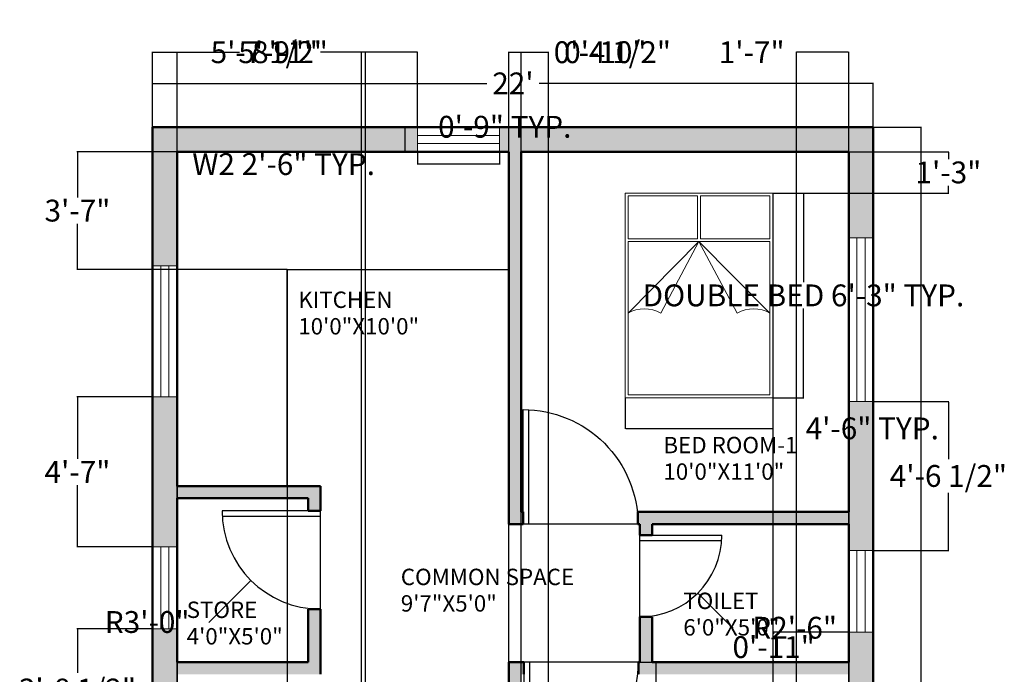
# Model space of a CAD drawing. Units: inches. Extents: x 23 to 387, y 67 to 650.
# Tile 3 of 3: x 23 to 384, y 410 to 650. Entities that reach past the tile are written whole.
import ezdxf

# ---------------------------------------------------------------- set-up
doc = ezdxf.new("R2010")
doc.units = ezdxf.units.IN
doc.header["$MEASUREMENT"] = 0
for name, color, linetype, lineweight in [('A-ANNO-DIMS', 4, 'Continuous', 18), ('A-AREA-IDEN', 4, 'Continuous', 25), ('A-DOOR', 41, 'Continuous', 25), ('A-FLOR-FIXT', 31, 'Continuous', 25), ('A-FURN', 31, 'Continuous', 18), ('A-GLAZ', 146, 'Continuous', 18), ('A-WALL', 240, 'Continuous', 50), ('A-WALL-PATT', 31, 'Continuous', 13)]:
    doc.layers.add(name, color=color, linetype=linetype, lineweight=lineweight)
doc.styles.get("Standard").update_dxf_attribs({"font": 'italic8.shx'})
doc.dimstyles.get("Standard").update_dxf_attribs({"dimtxt": 8, "dimasz": 0.18, "dimexe": 0.18, "dimexo": 0.0625, "dimgap": 0.09, "dimtad": 0, "dimtih": 1, "dimtoh": 1, "dimdec": 1, "dimzin": 0, "dimdsep": 46, "dimlunit": 3, "dimtxsty": 'Standard', "dimcen": 0.09, "dimadec": 0, "dimazin": 0, "dimtfac": 1, "dimtdec": 1, "dimtofl": 0, "dimtmove": 0, "dimatfit": 3, "dimfxl": 1, "dimtolj": 1, "dimtzin": 0, "dimarcsym": 0})

# ---------------------------------------------------------------- blocks, each defined once
blk = doc.blocks.new('*D4')
at = {"layer": 'A-ANNO-DIMS', "color": 0, "lineweight": -2, "transparency": 16777216}
for p, q in [((71.8, 610.61), (71.8, 626.8)), ((71.98, 626.62), (194.19, 626.62)), ((335.62, 626.62), (213.41, 626.62)), ((335.8, 610.61), (335.8, 626.8))]:
    blk.add_line(p, q, dxfattribs=at)
at = {"layer": 'A-ANNO-DIMS', "color": 0, "transparency": 16777216}
for points in [[(71.98, 626.65), (71.98, 626.59), (71.8, 626.62)], [(335.62, 626.65), (335.62, 626.59), (335.8, 626.62)]]:
    blk.add_solid(points, dxfattribs=at)
at = {"layer": 'Defpoints', "color": 0, "transparency": 16777216}
for p in [(335.8, 626.62), (71.8, 610.55), (335.8, 610.55)]:
    blk.add_point(p, dxfattribs=at)
at = {"layer": 'A-ANNO-DIMS', "color": 0, "transparency": 16777216, "insert": (203.8, 626.62), "char_height": 8, "attachment_point": 5}
blk.add_mtext("\\A1;22'", dxfattribs=at)
blk = doc.blocks.new('*D5')
at = {"layer": 'A-ANNO-DIMS', "color": 0, "lineweight": -2, "transparency": 16777216}
for p, q in [((335.86, 610.55), (353.42, 610.55)), ((353.24, 610.37), (353.24, 375.4)), ((353.24, 130.73), (353.24, 365.7)), ((335.86, 130.55), (353.42, 130.55))]:
    blk.add_line(p, q, dxfattribs=at)
at = {"layer": 'A-ANNO-DIMS', "color": 0, "transparency": 16777216}
for points in [[(353.21, 610.37), (353.27, 610.37), (353.24, 610.55)], [(353.21, 130.73), (353.27, 130.73), (353.24, 130.55)]]:
    blk.add_solid(points, dxfattribs=at)
at = {"layer": 'Defpoints', "color": 0, "transparency": 16777216}
for p in [(335.8, 610.55), (335.8, 130.55), (353.24, 130.55)]:
    blk.add_point(p, dxfattribs=at)
at = {"layer": 'A-ANNO-DIMS', "color": 0, "transparency": 16777216, "insert": (353.24, 370.55), "char_height": 8, "attachment_point": 5}
blk.add_mtext("\\A1;40'", dxfattribs=at)
blk = doc.blocks.new('BED-DOUBLE')
for p, q in [((26.5, 58.27), (26.5, 74)), ((27.5, 58.27), (27.5, 74)), ((1, 58.27), (26.5, 58.27)), ((27.5, 58.27), (53, 58.27)), ((1, 57.27), (53, 57.27)), ((27, 57.27), (1, 30.99)), ((13, 30.99), (27, 57.27)), ((27, 57.27), (53, 30.99)), ((41, 30.99), (27, 57.27))]:
    blk.add_line(p, q)
blk.add_lwpolyline([(54, 75), (0, 75), (0, 0), (54, 0)], close=True)
for points in [[(26.5, 74), (1, 74), (1, 58.27)], [(53, 58.27), (53, 74), (27.5, 74)], [(1, 57.27), (1, 1), (53, 1), (53, 57.27)]]:
    blk.add_lwpolyline(points)
for centre in [(7, 20.75), (47, 20.75)]:
    blk.add_arc(centre, 11.86, 59.6151, 120.3849)
blk = doc.blocks.new('DOOR-SWING-42IN')
for p, q in [((42, 42), (0, 42)), ((0, 42), (0, 0)), ((2, 42), (2, 0.05))]:
    blk.add_line(p, q)
blk.add_arc((0, 42), 42, 270, 0)
blk = doc.blocks.new('WIN-60IN')
for p, q in [((0, 0), (0, 60)), ((0, 60), (9, 60)), ((3, 0), (3, 60)), ((6, 0), (6, 60)), ((9, 60), (9, 0)), ((9, 0), (0, 0)), ((0, 0), (4.5, 0))]:
    blk.add_line(p, q)
blk = doc.blocks.new('WIN-30IN')
for p, q in [((0, 0), (0, 30)), ((0, 30), (9, 30)), ((3, 0), (3, 30)), ((6, 0), (6, 30)), ((9, 30), (9, 0)), ((9, 0), (0, 0)), ((0, 0), (4.5, 0))]:
    blk.add_line(p, q)
blk = doc.blocks.new('WIN-48IN')
for p, q in [((0, 0), (0, 48)), ((0, 48), (9, 48)), ((3, 0), (3, 48)), ((6, 0), (6, 48)), ((9, 48), (9, 0)), ((9, 0), (0, 0)), ((0, 0), (4.5, 0))]:
    blk.add_line(p, q)
blk = doc.blocks.new('*D14')
at = {"layer": 'A-ANNO-DIMS', "color": 0, "lineweight": -2, "transparency": 16777216}
for p, q in [((168.85, 601.49), (168.85, 596.87)), ((198.85, 601.49), (198.85, 596.87)), ((168.85, 597.05), (168.67, 597.05)), ((198.67, 597.05), (169.03, 597.05))]:
    blk.add_line(p, q, dxfattribs=at)
at = {"layer": 'A-ANNO-DIMS', "color": 0, "transparency": 16777216}
for points in [[(169.03, 597.08), (169.03, 597.02), (168.85, 597.05)], [(198.67, 597.08), (198.67, 597.02), (198.85, 597.05)]]:
    blk.add_solid(points, dxfattribs=at)
at = {"layer": 'Defpoints', "color": 0, "transparency": 16777216}
for p in [(168.85, 601.55), (198.85, 601.55), (168.85, 597.05)]:
    blk.add_point(p, dxfattribs=at)
at = {"layer": 'A-ANNO-DIMS', "color": 0, "transparency": 16777216, "insert": (119.81, 597.05), "char_height": 8, "attachment_point": 5}
blk.add_mtext('\\A1;W2 2\'-6" TYP.', dxfattribs=at)
blk = doc.blocks.new('*D15')
at = {"layer": 'A-ANNO-DIMS', "color": 0, "lineweight": -2, "transparency": 16777216}
for p, q in [((168.78, 610.55), (164.17, 610.55)), ((164.35, 610.55), (164.35, 610.73)), ((164.35, 610.73), (164.53, 610.73)), ((164.35, 601.73), (164.35, 610.37)), ((168.78, 601.55), (164.17, 601.55))]:
    blk.add_line(p, q, dxfattribs=at)
at = {"layer": 'A-ANNO-DIMS', "color": 0, "transparency": 16777216}
for points in [[(164.32, 610.37), (164.38, 610.37), (164.35, 610.55)], [(164.32, 601.73), (164.38, 601.73), (164.35, 601.55)]]:
    blk.add_solid(points, dxfattribs=at)
at = {"layer": 'Defpoints', "color": 0, "transparency": 16777216}
for p in [(164.35, 610.55), (168.85, 610.55), (168.85, 601.55)]:
    blk.add_point(p, dxfattribs=at)
at = {"layer": 'A-ANNO-DIMS', "color": 0, "transparency": 16777216, "insert": (200.81, 610.73), "char_height": 8, "attachment_point": 5}
blk.add_mtext('\\A1;0\'-9" TYP.', dxfattribs=at)
blk = doc.blocks.new('*D18')
at = {"layer": 'A-ANNO-DIMS', "color": 0, "lineweight": -2, "transparency": 16777216}
for p, q in [((299.01, 586.43), (310.38, 586.43)), ((310.2, 586.25), (310.2, 553.78)), ((310.2, 511.61), (310.2, 544.07)), ((299.01, 511.43), (310.38, 511.43))]:
    blk.add_line(p, q, dxfattribs=at)
at = {"layer": 'A-ANNO-DIMS', "color": 0, "transparency": 16777216}
for points in [[(310.17, 586.25), (310.23, 586.25), (310.2, 586.43)], [(310.17, 511.61), (310.23, 511.61), (310.2, 511.43)]]:
    blk.add_solid(points, dxfattribs=at)
at = {"layer": 'Defpoints', "color": 0, "transparency": 16777216}
for p in [(298.95, 586.43), (310.2, 586.43), (298.95, 511.43)]:
    blk.add_point(p, dxfattribs=at)
at = {"layer": 'A-ANNO-DIMS', "color": 0, "transparency": 16777216, "insert": (310.2, 548.93), "char_height": 8, "attachment_point": 5}
blk.add_mtext('\\A1;DOUBLE BED 6\'-3" TYP.', dxfattribs=at)
blk = doc.blocks.new('*D19')
at = {"layer": 'A-ANNO-DIMS', "color": 0, "lineweight": -2, "transparency": 16777216}
for p, q in [((244.95, 511.36), (244.95, 500)), ((298.95, 511.36), (298.95, 500)), ((245.13, 500.18), (298.77, 500.18)), ((298.95, 500.18), (299.13, 500.18))]:
    blk.add_line(p, q, dxfattribs=at)
at = {"layer": 'A-ANNO-DIMS', "color": 0, "transparency": 16777216}
for points in [[(245.13, 500.21), (245.13, 500.15), (244.95, 500.18)], [(298.77, 500.21), (298.77, 500.15), (298.95, 500.18)]]:
    blk.add_solid(points, dxfattribs=at)
at = {"layer": 'Defpoints', "color": 0, "transparency": 16777216}
for p in [(244.95, 511.43), (298.95, 511.43), (298.95, 500.18)]:
    blk.add_point(p, dxfattribs=at)
at = {"layer": 'A-ANNO-DIMS', "color": 0, "transparency": 16777216, "insert": (335.41, 500.18), "char_height": 8, "attachment_point": 5}
blk.add_mtext('\\A1;4\'-6" TYP.', dxfattribs=at)
blk = doc.blocks.new('*D21')
at = {"layer": 'A-ANNO-DIMS', "color": 0, "lineweight": -2, "transparency": 16777216}
for p, q in [((249.89, 414.55), (256.3, 414.55)), ((256.12, 414.37), (256.12, 398.4)), ((256.12, 372.73), (256.12, 388.7)), ((249.89, 372.55), (256.3, 372.55))]:
    blk.add_line(p, q, dxfattribs=at)
at = {"layer": 'A-ANNO-DIMS', "color": 0, "transparency": 16777216}
for points in [[(256.09, 414.37), (256.15, 414.37), (256.12, 414.55)], [(256.09, 372.73), (256.15, 372.73), (256.12, 372.55)]]:
    blk.add_solid(points, dxfattribs=at)
at = {"layer": 'Defpoints', "color": 0, "transparency": 16777216}
for p in [(249.82, 414.55), (256.12, 414.55), (249.82, 372.55)]:
    blk.add_point(p, dxfattribs=at)
at = {"layer": 'A-ANNO-DIMS', "color": 0, "transparency": 16777216, "insert": (256.12, 393.55), "char_height": 8, "attachment_point": 5}
blk.add_mtext('\\A1;3\'-6" TYP.', dxfattribs=at)
blk = doc.blocks.new('*D27')
at = {"layer": 'A-ANNO-DIMS', "color": 0, "lineweight": -2, "transparency": 16777216}
for p, q in [((71.8, 610.61), (71.8, 638.23)), ((71.98, 638.05), (103.66, 638.05)), ((168.67, 638.05), (136.98, 638.05)), ((168.85, 610.61), (168.85, 638.23))]:
    blk.add_line(p, q, dxfattribs=at)
at = {"layer": 'A-ANNO-DIMS', "color": 0, "transparency": 16777216}
for points in [[(71.98, 638.08), (71.98, 638.02), (71.8, 638.05)], [(168.67, 638.08), (168.67, 638.02), (168.85, 638.05)]]:
    blk.add_solid(points, dxfattribs=at)
at = {"layer": 'Defpoints', "color": 0, "transparency": 16777216}
for p in [(168.85, 638.05), (71.8, 610.55), (168.85, 610.55)]:
    blk.add_point(p, dxfattribs=at)
at = {"layer": 'A-ANNO-DIMS', "color": 0, "transparency": 16777216, "insert": (120.32, 638.05), "char_height": 8, "attachment_point": 5}
blk.add_mtext('\\A1;8\'-1"', dxfattribs=at)
blk = doc.blocks.new('*D29')
at = {"layer": 'A-ANNO-DIMS', "color": 0, "lineweight": -2, "transparency": 16777216}
for p, q in [((71.74, 511.71), (44.12, 511.71)), ((44.3, 511.53), (44.3, 489.07)), ((44.3, 456.92), (44.3, 479.37)), ((71.74, 456.74), (44.12, 456.74))]:
    blk.add_line(p, q, dxfattribs=at)
at = {"layer": 'A-ANNO-DIMS', "color": 0, "transparency": 16777216}
for points in [[(44.27, 511.53), (44.33, 511.53), (44.3, 511.71)], [(44.27, 456.92), (44.33, 456.92), (44.3, 456.74)]]:
    blk.add_solid(points, dxfattribs=at)
at = {"layer": 'Defpoints', "color": 0, "transparency": 16777216}
for p in [(71.8, 511.71), (44.3, 456.74), (71.8, 456.74)]:
    blk.add_point(p, dxfattribs=at)
at = {"layer": 'A-ANNO-DIMS', "color": 0, "transparency": 16777216, "insert": (44.3, 484.22), "char_height": 8, "attachment_point": 5}
blk.add_mtext('\\A1;4\'-7"', dxfattribs=at)
blk = doc.blocks.new('*D30')
at = {"layer": 'A-ANNO-DIMS', "color": 0, "lineweight": -2, "transparency": 16777216}
for p, q in [((71.74, 426.74), (44.12, 426.74)), ((44.3, 426.56), (44.3, 410.65)), ((44.3, 382.38), (44.3, 398.28)), ((71.74, 382.2), (44.12, 382.2))]:
    blk.add_line(p, q, dxfattribs=at)
at = {"layer": 'A-ANNO-DIMS', "color": 0, "transparency": 16777216}
for points in [[(44.27, 426.56), (44.33, 426.56), (44.3, 426.74)], [(44.27, 382.38), (44.33, 382.38), (44.3, 382.2)]]:
    blk.add_solid(points, dxfattribs=at)
at = {"layer": 'Defpoints', "color": 0, "transparency": 16777216}
for p in [(71.8, 426.74), (44.3, 382.2), (71.8, 382.2)]:
    blk.add_point(p, dxfattribs=at)
at = {"layer": 'A-ANNO-DIMS', "color": 0, "transparency": 16777216, "insert": (44.3, 404.47), "char_height": 8, "attachment_point": 5}
blk.add_mtext('\\A1;3\'-8 1/2"', dxfattribs=at)
blk = doc.blocks.new('*D33')
at = {"layer": 'A-ANNO-DIMS', "color": 0, "lineweight": -2, "transparency": 16777216}
for p, q in [((335.86, 510), (363.48, 510)), ((363.3, 509.82), (363.3, 488.93)), ((363.3, 455.67), (363.3, 476.56)), ((335.86, 455.49), (363.48, 455.49))]:
    blk.add_line(p, q, dxfattribs=at)
at = {"layer": 'A-ANNO-DIMS', "color": 0, "transparency": 16777216}
for points in [[(363.27, 509.82), (363.33, 509.82), (363.3, 510)], [(363.27, 455.67), (363.33, 455.67), (363.3, 455.49)]]:
    blk.add_solid(points, dxfattribs=at)
at = {"layer": 'Defpoints', "color": 0, "transparency": 16777216}
for p in [(335.8, 510), (335.8, 455.49), (363.3, 455.49)]:
    blk.add_point(p, dxfattribs=at)
at = {"layer": 'A-ANNO-DIMS', "color": 0, "transparency": 16777216, "insert": (363.3, 482.75), "char_height": 8, "attachment_point": 5}
blk.add_mtext('\\A1;4\'-6 1/2"', dxfattribs=at)
blk = doc.blocks.new('*D34')
at = {"layer": 'A-ANNO-DIMS', "color": 0, "lineweight": -2, "transparency": 16777216}
for p, q in [((326.74, 425.49), (299.12, 425.49)), ((299.3, 425.31), (299.3, 424.87)), ((299.3, 414.73), (299.3, 415.17)), ((326.74, 414.55), (299.12, 414.55))]:
    blk.add_line(p, q, dxfattribs=at)
at = {"layer": 'A-ANNO-DIMS', "color": 0, "transparency": 16777216}
for points in [[(299.27, 425.31), (299.33, 425.31), (299.3, 425.49)], [(299.27, 414.73), (299.33, 414.73), (299.3, 414.55)]]:
    blk.add_solid(points, dxfattribs=at)
at = {"layer": 'Defpoints', "color": 0, "transparency": 16777216}
for p in [(299.3, 425.49), (326.8, 425.49), (326.8, 414.55)]:
    blk.add_point(p, dxfattribs=at)
at = {"layer": 'A-ANNO-DIMS', "color": 0, "transparency": 16777216, "insert": (299.3, 420.02), "char_height": 8, "attachment_point": 5}
blk.add_mtext('\\A1;0\'-11"', dxfattribs=at)
blk = doc.blocks.new('*D37')
at = {"layer": 'A-ANNO-DIMS', "color": 0, "lineweight": -2, "transparency": 16777216}
for p, q in [((80.8, 139.61), (80.8, 638.23)), ((80.98, 638.05), (81.51, 638.05)), ((148.12, 638.05), (147.59, 638.05)), ((148.3, 139.61), (148.3, 638.23))]:
    blk.add_line(p, q, dxfattribs=at)
at = {"layer": 'A-ANNO-DIMS', "color": 0, "transparency": 16777216}
for points in [[(80.98, 638.08), (80.98, 638.02), (80.8, 638.05)], [(148.12, 638.08), (148.12, 638.02), (148.3, 638.05)]]:
    blk.add_solid(points, dxfattribs=at)
at = {"layer": 'Defpoints', "color": 0, "transparency": 16777216}
for p in [(148.3, 638.05), (80.8, 139.55), (148.3, 139.55)]:
    blk.add_point(p, dxfattribs=at)
at = {"layer": 'A-ANNO-DIMS', "color": 0, "transparency": 16777216, "insert": (114.55, 638.05), "char_height": 8, "attachment_point": 5}
blk.add_mtext('\\A1;5\'-7 1/2"', dxfattribs=at)
blk = doc.blocks.new('*D38')
at = {"layer": 'A-ANNO-DIMS', "color": 0, "lineweight": -2, "transparency": 16777216}
for p, q in [((80.8, 274.61), (80.8, 638.23)), ((80.98, 638.05), (97.28, 638.05)), ((149.58, 638.05), (133.27, 638.05)), ((149.76, 274.61), (149.76, 638.23))]:
    blk.add_line(p, q, dxfattribs=at)
at = {"layer": 'A-ANNO-DIMS', "color": 0, "transparency": 16777216}
for points in [[(80.98, 638.08), (80.98, 638.02), (80.8, 638.05)], [(149.58, 638.08), (149.58, 638.02), (149.76, 638.05)]]:
    blk.add_solid(points, dxfattribs=at)
at = {"layer": 'Defpoints', "color": 0, "transparency": 16777216}
for p in [(149.76, 638.05), (80.8, 274.55), (149.76, 274.55)]:
    blk.add_point(p, dxfattribs=at)
at = {"layer": 'A-ANNO-DIMS', "color": 0, "transparency": 16777216, "insert": (115.28, 638.05), "char_height": 8, "attachment_point": 5}
blk.add_mtext('\\A1;5\'-9"', dxfattribs=at)
blk = doc.blocks.new('*D39')
at = {"layer": 'A-ANNO-DIMS', "color": 0, "lineweight": -2, "transparency": 16777216}
for p, q in [((206.8, 192.11), (206.8, 638.23)), ((206.98, 638.05), (216.62, 638.05)), ((216.8, 192.11), (216.8, 638.23)), ((216.8, 638.05), (216.98, 638.05))]:
    blk.add_line(p, q, dxfattribs=at)
at = {"layer": 'A-ANNO-DIMS', "color": 0, "transparency": 16777216}
for points in [[(206.98, 638.08), (206.98, 638.02), (206.8, 638.05)], [(216.62, 638.08), (216.62, 638.02), (216.8, 638.05)]]:
    blk.add_solid(points, dxfattribs=at)
at = {"layer": 'Defpoints', "color": 0, "transparency": 16777216}
for p in [(216.8, 638.05), (206.8, 192.05), (216.8, 192.05)]:
    blk.add_point(p, dxfattribs=at)
at = {"layer": 'A-ANNO-DIMS', "color": 0, "transparency": 16777216, "insert": (237.64, 638.05), "char_height": 8, "attachment_point": 5}
blk.add_mtext('\\A1;0\'-10"', dxfattribs=at)
blk = doc.blocks.new('*D40')
at = {"layer": 'A-ANNO-DIMS', "color": 0, "lineweight": -2, "transparency": 16777216}
for p, q in [((80.8, 601.49), (80.8, 78.87)), ((121.14, 558.4), (121.14, 78.87)), ((80.8, 79.05), (80.62, 79.05)), ((120.96, 79.05), (80.98, 79.05))]:
    blk.add_line(p, q, dxfattribs=at)
at = {"layer": 'A-ANNO-DIMS', "color": 0, "transparency": 16777216}
for points in [[(80.98, 79.08), (80.98, 79.02), (80.8, 79.05)], [(120.96, 79.08), (120.96, 79.02), (121.14, 79.05)]]:
    blk.add_solid(points, dxfattribs=at)
at = {"layer": 'Defpoints', "color": 0, "transparency": 16777216}
for p in [(80.8, 601.55), (121.14, 558.46), (80.8, 79.05)]:
    blk.add_point(p, dxfattribs=at)
at = {"layer": 'A-ANNO-DIMS', "color": 0, "transparency": 16777216, "insert": (47.39, 79.05), "char_height": 8, "attachment_point": 5}
blk.add_mtext('\\A1;3\'-4 1/2"', dxfattribs=at)
blk = doc.blocks.new('*D41')
at = {"layer": 'A-ANNO-DIMS', "color": 0, "lineweight": -2, "transparency": 16777216}
for p, q in [((80.74, 601.55), (44.12, 601.55)), ((44.3, 601.37), (44.3, 584.86)), ((44.3, 558.64), (44.3, 575.15)), ((121.07, 558.46), (44.12, 558.46))]:
    blk.add_line(p, q, dxfattribs=at)
at = {"layer": 'A-ANNO-DIMS', "color": 0, "transparency": 16777216}
for points in [[(44.27, 601.37), (44.33, 601.37), (44.3, 601.55)], [(44.27, 558.64), (44.33, 558.64), (44.3, 558.46)]]:
    blk.add_solid(points, dxfattribs=at)
at = {"layer": 'Defpoints', "color": 0, "transparency": 16777216}
for p in [(80.8, 601.55), (44.3, 558.46), (121.14, 558.46)]:
    blk.add_point(p, dxfattribs=at)
at = {"layer": 'A-ANNO-DIMS', "color": 0, "transparency": 16777216, "insert": (44.3, 580), "char_height": 8, "attachment_point": 5}
blk.add_mtext('\\A1;3\'-7"', dxfattribs=at)
blk = doc.blocks.new('*D42')
at = {"layer": 'A-ANNO-DIMS', "color": 0, "lineweight": -2, "transparency": 16777216}
for p, q in [((202.3, 274.61), (202.3, 638.23)), ((202.48, 638.05), (206.62, 638.05)), ((206.8, 274.61), (206.8, 638.23)), ((206.8, 638.05), (206.98, 638.05))]:
    blk.add_line(p, q, dxfattribs=at)
at = {"layer": 'A-ANNO-DIMS', "color": 0, "transparency": 16777216}
for points in [[(202.48, 638.08), (202.48, 638.02), (202.3, 638.05)], [(206.62, 638.08), (206.62, 638.02), (206.8, 638.05)]]:
    blk.add_solid(points, dxfattribs=at)
at = {"layer": 'Defpoints', "color": 0, "transparency": 16777216}
for p in [(206.8, 638.05), (202.3, 274.55), (206.8, 274.55)]:
    blk.add_point(p, dxfattribs=at)
at = {"layer": 'A-ANNO-DIMS', "color": 0, "transparency": 16777216, "insert": (240.21, 638.05), "char_height": 8, "attachment_point": 5}
blk.add_mtext('\\A1;0\'-4 1/2"', dxfattribs=at)
blk = doc.blocks.new('*D43')
at = {"layer": 'A-ANNO-DIMS', "color": 0, "lineweight": -2, "transparency": 16777216}
for p, q in [((326.8, 601.49), (326.8, 78.87)), ((298.95, 586.36), (298.95, 78.87)), ((298.95, 79.05), (298.77, 79.05)), ((326.62, 79.05), (299.13, 79.05))]:
    blk.add_line(p, q, dxfattribs=at)
at = {"layer": 'A-ANNO-DIMS', "color": 0, "transparency": 16777216}
for points in [[(299.13, 79.08), (299.13, 79.02), (298.95, 79.05)], [(326.62, 79.08), (326.62, 79.02), (326.8, 79.05)]]:
    blk.add_solid(points, dxfattribs=at)
at = {"layer": 'Defpoints', "color": 0, "transparency": 16777216}
for p in [(326.8, 601.55), (298.95, 586.43), (298.95, 79.05)]:
    blk.add_point(p, dxfattribs=at)
at = {"layer": 'A-ANNO-DIMS', "color": 0, "transparency": 16777216, "insert": (280.78, 79.05), "char_height": 8, "attachment_point": 5}
blk.add_mtext('\\A1;2\'-4"', dxfattribs=at)
blk = doc.blocks.new('*D44')
at = {"layer": 'A-ANNO-DIMS', "color": 0, "lineweight": -2, "transparency": 16777216}
for p, q in [((326.86, 601.55), (363.48, 601.55)), ((363.3, 601.37), (363.3, 598.84)), ((363.3, 586.61), (363.3, 589.14)), ((299.01, 586.43), (363.48, 586.43))]:
    blk.add_line(p, q, dxfattribs=at)
at = {"layer": 'A-ANNO-DIMS', "color": 0, "transparency": 16777216}
for points in [[(363.27, 601.37), (363.33, 601.37), (363.3, 601.55)], [(363.27, 586.61), (363.33, 586.61), (363.3, 586.43)]]:
    blk.add_solid(points, dxfattribs=at)
at = {"layer": 'Defpoints', "color": 0, "transparency": 16777216}
for p in [(326.8, 601.55), (298.95, 586.43), (363.3, 586.43)]:
    blk.add_point(p, dxfattribs=at)
at = {"layer": 'A-ANNO-DIMS', "color": 0, "transparency": 16777216, "insert": (363.3, 593.99), "char_height": 8, "attachment_point": 5}
blk.add_mtext('\\A1;1\'-3"', dxfattribs=at)
blk = doc.blocks.new('*D45')
at = {"layer": 'A-ANNO-DIMS', "color": 0, "lineweight": -2, "transparency": 16777216}
for p, q in [((307.71, 638.05), (307.53, 638.05)), ((307.71, 290.5), (307.71, 638.23)), ((326.62, 638.05), (307.89, 638.05)), ((326.8, 274.61), (326.8, 638.23))]:
    blk.add_line(p, q, dxfattribs=at)
at = {"layer": 'A-ANNO-DIMS', "color": 0, "transparency": 16777216}
for points in [[(307.89, 638.08), (307.89, 638.02), (307.71, 638.05)], [(326.62, 638.08), (326.62, 638.02), (326.8, 638.05)]]:
    blk.add_solid(points, dxfattribs=at)
at = {"layer": 'Defpoints', "color": 0, "transparency": 16777216}
for p in [(307.71, 638.05), (307.71, 290.44), (326.8, 274.55)]:
    blk.add_point(p, dxfattribs=at)
at = {"layer": 'A-ANNO-DIMS', "color": 0, "transparency": 16777216, "insert": (291.25, 638.05), "char_height": 8, "attachment_point": 5}
blk.add_mtext('\\A1;1\'-7"', dxfattribs=at)
blk = doc.blocks.new('*D48')
at = {"layer": 'A-ANNO-DIMS', "color": 0, "lineweight": -2, "transparency": 16777216}
for p, q in [((133.21, 469.95), (133.39, 469.95)), ((133.3, 469.86), (133.3, 470.04)), ((92.57, 429.22), (107.72, 444.36)), ((92.39, 429.22), (92.57, 429.22))]:
    blk.add_line(p, q, dxfattribs=at)
at = {"layer": 'A-ANNO-DIMS', "color": 0, "transparency": 16777216}
blk.add_solid([(107.69, 444.39), (107.74, 444.34), (107.84, 444.49)], dxfattribs=at)
at = {"layer": 'Defpoints', "color": 0, "transparency": 16777216}
for p in [(133.3, 469.95), (107.84, 444.49)]:
    blk.add_point(p, dxfattribs=at)
at = {"layer": 'A-ANNO-DIMS', "color": 0, "transparency": 16777216, "insert": (69.82, 429.22), "char_height": 8, "attachment_point": 5}
blk.add_mtext('\\A1;R3\'-0"', dxfattribs=at)
blk = doc.blocks.new('*D49')
at = {"layer": 'A-ANNO-DIMS', "color": 0, "lineweight": -2, "transparency": 16777216}
for p, q in [((250.21, 461.06), (250.39, 461.06)), ((250.3, 460.97), (250.3, 461.15)), ((284.24, 427.12), (271.64, 439.72)), ((284.42, 427.12), (284.24, 427.12))]:
    blk.add_line(p, q, dxfattribs=at)
at = {"layer": 'A-ANNO-DIMS', "color": 0, "transparency": 16777216}
blk.add_solid([(271.66, 439.74), (271.62, 439.7), (271.51, 439.85)], dxfattribs=at)
at = {"layer": 'Defpoints', "color": 0, "transparency": 16777216}
for p in [(250.3, 461.06), (271.51, 439.85)]:
    blk.add_point(p, dxfattribs=at)
at = {"layer": 'A-ANNO-DIMS', "color": 0, "transparency": 16777216, "insert": (306.99, 427.12), "char_height": 8, "attachment_point": 5}
blk.add_mtext('\\A1;R2\'-6"', dxfattribs=at)

msp = doc.modelspace()

# ---------------------------------------------------------------- hatches: boundary and pattern name
at = {"layer": 'A-WALL-PATT'}
h = msp.add_hatch(color=256, dxfattribs=at)
h.dxf.hatch_style = 1
h.paths.add_polyline_path([(80.8, 601.55), (168.85, 601.55), (168.85, 610.55), (71.8, 610.55), (71.8, 559.71), (80.8, 559.71)])
h.paths.add_polyline_path([(335.8, 610.55), (198.85, 610.55), (198.85, 601.55), (202.3, 601.55), (202.3, 481.55), (202.3, 465.05), (207.59, 465.05), (207.59, 469.55), (206.8, 469.55), (206.8, 601.55), (326.8, 601.55), (326.8, 570), (331.3, 570), (335.8, 570)])
h.paths.add_polyline_path([(335.8, 510), (326.8, 510), (326.8, 469.55), (249.59, 469.55), (249.59, 465.05), (250.3, 465.05), (250.3, 461.06), (254.8, 461.06), (254.8, 465.05), (326.8, 465.05), (326.8, 455.49), (335.8, 455.49)])
h.paths.add_polyline_path([(335.8, 425.49), (326.8, 425.49), (326.8, 414.55), (254.8, 414.55), (254.8, 431.06), (250.3, 431.06), (250.3, 414.55), (249.82, 414.55), (249.82, 410.05), (326.8, 410.05), (326.8, 362.57), (335.8, 362.57)])
h.paths.add_polyline_path([(335.8, 302.57), (326.8, 302.57), (326.8, 274.55), (206.8, 274.55), (206.8, 410.05), (207.82, 410.05), (207.82, 414.55), (202.3, 414.55), (202.3, 274.55), (197.76, 274.55), (197.76, 270.05), (326.8, 270.05), (326.8, 253.25), (335.8, 253.25)])
h.paths.add_polyline_path([(335.8, 217.25), (326.8, 217.25), (326.8, 192.05), (202.3, 192.05), (202.3, 139.55), (196.3, 139.55), (196.3, 130.55), (206.8, 130.55), (206.8, 187.55), (335.8, 187.55)])
h.paths.add_polyline_path([(80.8, 203.04), (71.8, 203.04), (71.8, 130.55), (148.3, 130.55), (148.3, 139.55), (80.8, 139.55)])
h.paths.add_polyline_path([(80.8, 322.2), (71.8, 322.2), (71.8, 251.04), (80.8, 251.04), (80.8, 270.05), (149.76, 270.05), (149.76, 274.55), (80.8, 274.55)])
h.paths.add_polyline_path([(80.8, 410.05), (133.3, 410.05), (133.3, 433.95), (128.8, 433.95), (128.8, 414.55), (80.8, 414.55), (80.8, 426.74), (71.8, 426.74), (71.8, 382.2), (80.8, 382.2)])
h.paths.add_polyline_path([(133.3, 479.05), (80.8, 479.05), (80.8, 511.71), (71.8, 511.71), (71.8, 456.74), (80.8, 456.74), (80.8, 474.55), (128.8, 474.55), (128.8, 469.95), (133.3, 469.95)])
h.paths.add_polyline_path([(82.53, 419.2), (134.1, 419.2), (134.1, 429.92), (82.53, 429.92)], flags=9)

# ---------------------------------------------------------------- linework, layer by layer
at = {"layer": 'A-DOOR'}
for p, q in [((133.3, 469.95), (97.3, 469.95)), ((133.3, 433.95), (133.3, 469.95)), ((133.3, 467.95), (97.35, 467.95)), ((250.3, 431.06), (250.3, 461.06)), ((250.3, 461.06), (280.3, 461.06)), ((250.3, 459.06), (280.23, 459.06))]:
    msp.add_line(p, q, dxfattribs=at)
for centre, radius, start, end in [((133.3, 469.95), 36, 180, 270), ((250.3, 461.06), 30, 270, 0)]:
    msp.add_arc(centre, radius, start, end, dxfattribs=at)
at = {"layer": 'A-FLOR-FIXT'}
for p, q in [((121.14, 479.05), (121.14, 558.46)), ((121.14, 558.46), (202.3, 558.46))]:
    msp.add_line(p, q, dxfattribs=at)
at = {"layer": 'A-WALL'}
for p, q in [((335.8, 610.55), (71.8, 610.55)), ((71.8, 610.55), (71.8, 130.55)), ((335.8, 130.55), (335.8, 610.55)), ((80.8, 601.55), (80.8, 479.05)), ((202.3, 601.55), (80.8, 601.55)), ((202.3, 481.55), (202.3, 601.55)), ((326.8, 601.55), (206.8, 601.55)), ((206.8, 469.55), (206.8, 601.55)), ((326.8, 469.55), (326.8, 601.55)), ((202.3, 465.05), (202.3, 481.55)), ((80.8, 479.05), (133.3, 479.05)), ((133.3, 479.05), (133.3, 469.95)), ((80.8, 474.55), (80.8, 414.55)), ((80.8, 474.55), (128.8, 474.55)), ((128.8, 474.55), (128.8, 469.95)), ((128.8, 469.95), (133.3, 469.95)), ((207.59, 469.55), (206.8, 469.55)), ((207.59, 465.05), (207.59, 469.55)), ((326.8, 469.55), (249.59, 469.55)), ((249.59, 465.05), (249.59, 469.55)), ((207.59, 465.05), (202.3, 465.05)), ((250.3, 465.05), (249.59, 465.05)), ((250.3, 461.06), (250.3, 465.05)), ((326.8, 465.05), (254.8, 465.05)), ((254.8, 461.06), (254.8, 465.05)), ((326.8, 414.55), (326.8, 465.05)), ((250.3, 461.06), (254.8, 461.06)), ((128.8, 433.95), (133.3, 433.95)), ((128.8, 433.95), (128.8, 414.55)), ((133.3, 433.95), (133.3, 410.05)), ((250.3, 414.55), (250.3, 431.06)), ((250.3, 431.06), (254.8, 431.06)), ((254.8, 414.55), (254.8, 431.06)), ((80.8, 414.55), (128.8, 414.55)), ((202.3, 414.55), (207.82, 414.55)), ((202.3, 274.55), (202.3, 414.55)), ((207.82, 414.55), (207.82, 410.05)), ((249.82, 414.55), (249.82, 410.05)), ((249.82, 414.55), (250.3, 414.55)), ((254.8, 414.55), (326.8, 414.55))]:
    msp.add_line(p, q, dxfattribs=at)

# ---------------------------------------------------------------- block references
at = {"layer": 'A-DOOR', "extrusion": (0, 0, -1), "zscale": -1, "rotation": 180}
msp.add_blockref('DOOR-SWING-42IN', (-207.59, 507.05), dxfattribs=at)
at = {"layer": 'A-DOOR'}
msp.add_blockref('DOOR-SWING-42IN', (207.82, 372.55), dxfattribs=at)
at = {"layer": 'A-FURN'}
msp.add_blockref('BED-DOUBLE', (244.95, 511.43), dxfattribs=at)
at = {"layer": 'A-GLAZ', "rotation": 90.00000000000028}
msp.add_blockref('WIN-30IN', (198.85, 601.55), dxfattribs=at)
at = {"layer": 'A-GLAZ', "extrusion": (0, 0, -1), "zscale": -1, "rotation": 180}
msp.add_blockref('WIN-60IN', (-326.8, 570), dxfattribs=at)
at = {"layer": 'A-GLAZ'}
for name, p in [('WIN-48IN', (71.8, 511.71)), ('WIN-30IN', (71.8, 426.73)), ('WIN-30IN', (326.8, 425.49))]:
    msp.add_blockref(name, p, dxfattribs=at)

# ---------------------------------------------------------------- texts
at = {"layer": 'A-AREA-IDEN'}
for s, p in [('KITCHEN', (125.18, 544.33)), ('10\'0"X10\'0"', (125.18, 534.61)), ('BED ROOM-1', (258.92, 491.07)), ('10\'0"X11\'0"', (258.92, 481.35)), ('COMMON SPACE', (162.73, 442.75)), ('TOILET', (266.2, 433.98)), ('STORE', (84.31, 430.7)), ('9\'7"X5\'0"', (162.73, 433.04)), ('6\'0"X5\'0"', (266.2, 424.26)), ('4\'0"X5\'0"', (84.31, 420.99))]:
    msp.add_text(s, height=6, dxfattribs=at).set_placement(p)

# ---------------------------------------------------------------- dimensions: what is measured, and where the dimension line sits
at = {"layer": 'A-ANNO-DIMS'}
for base, p1, p2, override, picture, middle in [((148.3, 638.05), (80.8, 139.55), (148.3, 139.55), {"dimdec": 1, "dimlfac": 1, "dimrnd": 0, "dimzin": 1, "dimdsep": 46, "dimlunit": 4, "dimfrac": 2}, '*D37', (114.55, 638.05)), ((206.8, 638.05), (202.3, 274.55), (206.8, 274.55), {"dimdec": 1, "dimlfac": 1, "dimrnd": 0, "dimzin": 1, "dimdsep": 46, "dimlunit": 4, "dimfrac": 2}, '*D42', (240.21, 638.05)), ((168.8451, 638.049), (71.7992, 610.549), (168.8451, 610.549), {"dimdec": 1, "dimlfac": 1, "dimrnd": 0, "dimzin": 1, "dimdsep": 46, "dimlunit": 4, "dimfrac": 2}, '*D27', (120.3222, 638.049)), ((149.76, 638.05), (80.8, 274.55), (149.76, 274.55), {"dimdec": 1, "dimlfac": 1, "dimrnd": 0, "dimzin": 1, "dimdsep": 46, "dimlunit": 4, "dimfrac": 2}, '*D38', (115.28, 638.05)), ((216.8, 638.05), (206.8, 192.05), (216.8, 192.05), {"dimdec": 1, "dimlfac": 1, "dimrnd": 0, "dimzin": 1, "dimdsep": 46, "dimlunit": 4, "dimfrac": 2}, '*D39', (237.64, 638.05)), ((307.71, 638.05), (326.8, 274.55), (307.71, 290.44), {"dimdec": 1, "dimlfac": 1, "dimrnd": 0, "dimzin": 1, "dimdsep": 46, "dimlunit": 4, "dimfrac": 2}, '*D45', (291.25, 638.05)), ((335.8, 626.62), (71.8, 610.55), (335.8, 610.55), {"dimclrd": 0, "dimclre": 0, "dimclrt": 0}, '*D4', (203.8, 626.62)), ((80.8, 79.05), (121.14, 558.46), (80.8, 601.55), {"dimdec": 1, "dimlfac": 1, "dimrnd": 0, "dimzin": 1, "dimdsep": 46, "dimlunit": 4, "dimfrac": 2}, '*D40', (47.39, 79.05)), ((298.9524, 79.049), (326.7992, 601.549), (298.9524, 586.4268), {"dimdec": 1, "dimlfac": 1, "dimrnd": 0, "dimzin": 1, "dimdsep": 46, "dimlunit": 4, "dimfrac": 2}, '*D43', (280.7776, 79.049))]:
    dim = msp.add_linear_dim(base=base, p1=p1, p2=p2, dimstyle='Standard', override=override, dxfattribs=at)
    dim.commit()
    dim.dimension.update_dxf_attribs({"geometry": picture, "text_midpoint": middle})
for base, p1, p2, angle, text, picture, middle in [((164.35, 610.55), (168.85, 601.55), (168.85, 610.55), 90, '<> TYP.', '*D15', (200.81, 610.73)), ((168.85, 597.05), (198.85, 601.55), (168.85, 601.55), 180, 'W2 <> TYP.', '*D14', (119.81, 597.05)), ((310.2, 586.43), (298.95, 511.43), (298.95, 586.43), 90, 'DOUBLE BED <> TYP.', '*D18', (310.2, 548.93)), ((256.12, 414.55), (249.82, 372.55), (249.82, 414.55), 90, '<> TYP.', '*D21', (256.12, 393.55))]:
    dim = msp.add_linear_dim(base=base, p1=p1, p2=p2, angle=angle, text=text, dimstyle='Standard', override={"dimdec": 1, "dimlfac": 1, "dimrnd": 0, "dimzin": 1, "dimdsep": 46, "dimlunit": 4, "dimfrac": 2}, dxfattribs=at)
    dim.commit()
    dim.dimension.update_dxf_attribs({"geometry": picture, "text_midpoint": middle})
for base, p1, p2, override, picture, middle in [((353.24, 130.55), (335.8, 610.55), (335.8, 130.55), {"dimclrd": 0, "dimclre": 0, "dimclrt": 0}, '*D5', (353.24, 370.55)), ((44.3, 558.46), (80.8, 601.55), (121.14, 558.46), {"dimdec": 1, "dimlfac": 1, "dimrnd": 0, "dimzin": 1, "dimdsep": 46, "dimlunit": 4, "dimfrac": 2}, '*D41', (44.3, 580)), ((363.3, 586.43), (326.8, 601.55), (298.95, 586.43), {"dimdec": 1, "dimlfac": 1, "dimrnd": 0, "dimzin": 1, "dimdsep": 46, "dimlunit": 4, "dimfrac": 2}, '*D44', (363.3, 593.99)), ((44.3, 456.74), (71.8, 511.71), (71.8, 456.74), {"dimdec": 1, "dimlfac": 1, "dimrnd": 0, "dimzin": 1, "dimdsep": 46, "dimlunit": 4, "dimfrac": 2}, '*D29', (44.3, 484.22)), ((363.3, 455.49), (335.8, 510), (335.8, 455.49), {"dimdec": 1, "dimlfac": 1, "dimrnd": 0, "dimzin": 1, "dimdsep": 46, "dimlunit": 4, "dimfrac": 2}, '*D33', (363.3, 482.75)), ((44.3, 382.2), (71.8, 426.74), (71.8, 382.2), {"dimdec": 1, "dimlfac": 1, "dimrnd": 0, "dimzin": 1, "dimdsep": 46, "dimlunit": 4, "dimfrac": 2}, '*D30', (44.3, 404.47)), ((299.3, 425.49), (326.8, 414.55), (326.8, 425.49), {"dimdec": 1, "dimlfac": 1, "dimrnd": 0, "dimzin": 1, "dimdsep": 46, "dimlunit": 4, "dimfrac": 2}, '*D34', (299.3, 420.02))]:
    dim = msp.add_linear_dim(base=base, p1=p1, p2=p2, angle=90, dimstyle='Standard', override=override, dxfattribs=at)
    dim.commit()
    dim.dimension.update_dxf_attribs({"geometry": picture, "text_midpoint": middle})
dim = msp.add_linear_dim(base=(298.95, 500.18), p1=(244.95, 511.43), p2=(298.95, 511.43), text='<> TYP.', dimstyle='Standard', override={"dimdec": 1, "dimlfac": 1, "dimrnd": 0, "dimzin": 1, "dimdsep": 46, "dimlunit": 4, "dimfrac": 2}, dxfattribs=at)
dim.commit()
dim.dimension.update_dxf_attribs({"geometry": '*D19', "text_midpoint": (335.41, 500.18)})
for center, mpoint, picture, middle in [((133.3, 469.95), (107.84, 444.49), '*D48', (69.82, 429.22)), ((250.3, 461.06), (271.51, 439.85), '*D49', (306.99, 427.12))]:
    dim = msp.add_radius_dim(center=center, mpoint=mpoint, dimstyle='Standard', override={"dimdec": 1, "dimlfac": 1, "dimrnd": 0, "dimzin": 1, "dimdsep": 46, "dimlunit": 4, "dimfrac": 2}, dxfattribs=at)
    dim.commit()
    dim.dimension.update_dxf_attribs({"geometry": picture, "text_midpoint": middle, "dimtype": 164})

doc.saveas('drawing.dxf')
